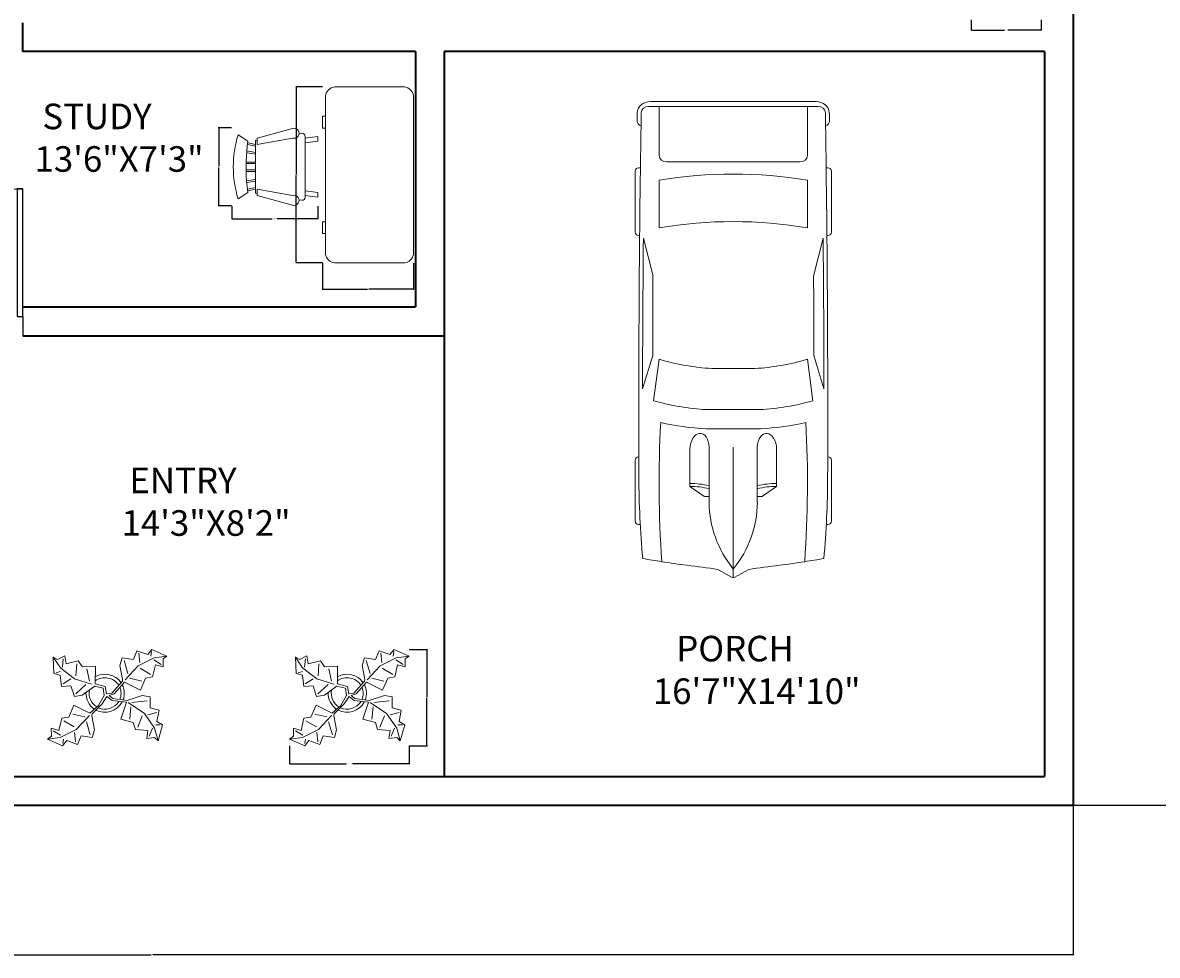
# Model space of a CAD drawing. Units: inches. Extents: x -1138 to 192, y 31 to 760.
# Tile 2 of 6: x -843 to -488, y 31 to 323. Entities that reach past the tile are written whole.
import ezdxf

# ---------------------------------------------------------------- set-up
doc = ezdxf.new("R2010")
doc.units = ezdxf.units.IN
doc.header["$MEASUREMENT"] = 0
for name, color, linetype, lineweight in [('A-ANNO-DIMS', 2, 'Continuous', 18), ('A-AREA-IDEN', 7, 'Continuous', 18), ('A-DOOR', 3, 'Continuous', 25), ('A-FURN', 8, 'Continuous', 18), ('A-SITE-VEHI', 8, 'Continuous', 13), ('A-WALL', 7, 'Continuous', 35), ('L-PLNT', 94, 'Continuous', 18)]:
    doc.layers.add(name, color=color, linetype=linetype, lineweight=lineweight)
doc.styles.get("Standard").update_dxf_attribs({"font": 'arial.ttf'})
doc.dimstyles.get("Standard").update_dxf_attribs({"dimtxt": 0.18, "dimasz": 0.18, "dimexe": 0.18, "dimexo": 0.0625, "dimgap": 0.09, "dimtad": 0, "dimtih": 1, "dimtoh": 1, "dimdec": 1, "dimzin": 0, "dimdsep": 46, "dimlunit": 4, "dimtxsty": 'Standard', "dimcen": 0.09, "dimadec": 0, "dimazin": 0, "dimtfac": 1, "dimtdec": 1, "dimtofl": 0, "dimtmove": 0, "dimatfit": 3, "dimfxl": 1, "dimtolj": 1, "dimtzin": 0, "dimarcsym": 0})

# ---------------------------------------------------------------- blocks, each defined once
blk = doc.blocks.new('*U9')
for p, q in [((0, 0), (0, -6)), ((40, 0), (40, -6))]:
    blk.add_line(p, q)
blk.add_lwpolyline([(0, 0), (0, 40), (1.75, 40), (1.75, 0)], close=True)
blk.add_arc((0, 0), 40, 0, 90)
blk = doc.blocks.new('*U11')
for p, q in [((536, 950), (536, 936)), ((1182, 988), (568, 988)), ((1214, 950), (1214, 950)), ((3440, 942), (3440, 950)), ((3472, 988), (4087, 988)), ((4119, 950), (4119, 934)), ((1779, 801), (2195, 746)), ((2235, 810), (1899, 912)), ((3412, 904), (3030, 807)), ((4736, -851), (4736, 851)), ((4785, -832), (4785, 832)), ((3516, 746), (3994, 746)), ((4736, 746), (4242, 746)), ((4179, 670), (4179, -670)), ((820, 295), (918, 436)), ((918, 436), (1294, 436)), ((756, 241), (1313, 241)), ((816, 241), (816, 283)), ((1496, -274), (1496, 274)), ((1690, -267), (1690, 267)), ((4736, -267), (4736, 267)), ((83, 156), (3, 10)), ((2102, 216), (2102, -216)), ((0, 0), (1313, 0)), ((3, -10), (83, -156)), ((756, -241), (1313, -241)), ((816, -241), (816, -283)), ((820, -295), (918, -436)), ((918, -436), (1294, -436)), ((2195, -746), (1779, -801)), ((3994, -746), (3516, -746)), ((4242, -746), (4736, -746)), ((2235, -810), (1899, -912)), ((3412, -904), (3030, -807)), ((536, -950), (536, -936)), ((1182, -988), (568, -988)), ((1214, -950), (1214, -950)), ((3440, -942), (3440, -950)), ((3472, -988), (4087, -988)), ((4119, -950), (4119, -934))]:
    blk.add_line(p, q)
for centre, major_axis, ratio, start_param, end_param in [((1046, -12468), (0, 13417), 0.842304, 0.00281, 0.075598), ((568, 950), (0, -37.6), 0.842304, 3.141593, 4.712389), ((1638, -268113), (0, 269063), 0.842304, -0.013397, 0.002797), ((1182, 950), (0, 37.6), 0.842304, -1.570796, 0), ((3472, 950), (0, -37.6), 0.842304, 3.141593, 4.712389), ((4087, 950), (0, 37.6), 0.842304, -1.570796, 0), ((4588, 910), (0, 56.4), 0.842304, -0.013017, 1.249894), ((1638, -268131), (0, 269121), 0.842304, -0.013397, -0.013017), ((4673, 851), (0, -75.2), 0.842304, 1.570796, 3.128196), ((4673, 832), (0, -133), 0.842304, 1.570796, 3.128196), ((6757, -699), (0, 7958), 0.842304, 1.367076, 1.39176), ((3436, 137), (0, 2077), 0.842304, 1.245306, 1.50788), ((1638, -268113), (0, -269025), 0.842304, 3.133765, 3.140441), ((2433, -93125), (0, -93935), 0.842304, 3.134049, 3.144098), ((6583, -699), (0, -7755), 0.842304, 4.528606, 4.561838), ((952, -15087), (0, -15833), 0.842304, 3.096046, 3.200911), ((3414, 137), (0, -2280), 0.842304, 4.449482, 4.652344), ((3800, 71), (0, -2021), 0.842304, 4.372215, 4.640744), ((434, 0), (0, 3734), 0.842304, 4.511394, 4.913384), ((912, 0), (0, 3734), 0.842304, 4.511394, 4.913384), ((4242, 670), (0, 75.2), 0.842304, 0, 1.570796), ((-5194, 1331), (0, -6374), 0.842304, 1.385369, 1.434372), ((331, 432), (0, 696), 0.842304, 4.435146, 4.718221), ((361, 432), (0, 696), 0.842304, 4.435146, 4.718221), ((1290, 339), (161, -9), 0.603834, -1.395552, 1.581315), ((756, -1185), (0, 1427), 0.842304, 0, 0.590319), ((832, 283), (0, 18.8), 0.842304, 0.879714, 1.570796), ((16, 0), (0, -18.8), 0.842304, 4.131459, 5.293319), ((756, 1185), (0, 1427), 0.842304, 2.551274, 3.141593), ((-5194, -1331), (0, 6374), 0.842304, -1.434372, -1.385369), ((3800, -71), (0, -2021), 0.842304, -1.499151, -1.230623), ((832, -283), (0, -18.8), 0.842304, 4.712389, 5.403472), ((331, -432), (0, -696), 0.842304, 1.564964, 1.848039), ((361, -432), (0, -696), 0.842304, 1.564964, 1.848039), ((3414, -137), (0, -2280), 0.842304, -1.510751, -1.307889), ((3436, -137), (0, -2077), 0.842304, -1.50788, -1.245306), ((6583, 699), (0, 7755), 0.842304, 1.721348, 1.754579), ((4242, -670), (0, -75.2), 0.842304, 4.712389, 6.283185), ((6757, 699), (0, 7958), 0.842304, 1.749832, 1.774517), ((952, 15087), (0, -15833), 0.842304, -0.059319, 0.045547), ((1046, 12468), (0, -13417), 0.842304, -0.075598, -0.00281), ((1638, 268113), (0, -269025), 0.842304, 0.001152, 0.007828), ((2433, 93125), (0, -93935), 0.842304, -0.002505, 0.007544), ((4673, -851), (0, 75.2), 0.842304, 3.15499, 4.712389), ((4673, -832), (0, -133), 0.842304, 0.013397, 1.570796), ((568, -950), (0, 37.6), 0.842304, 1.570796, 3.141593), ((1638, 268113), (0, 269063), 0.842304, 3.138796, 3.15499), ((1182, -950), (0, -37.6), 0.842304, 0, 1.570796), ((3472, -950), (0, -37.6), 0.842304, -1.570796, 0), ((4087, -950), (0, 37.6), 0.842304, 3.141593, 4.712389), ((4588, -910), (0, -56.4), 0.842304, -1.249894, 0.013017), ((1638, 268131), (0, 269121), 0.842304, 3.15461, 3.15499)]:
    blk.add_ellipse(centre, major_axis=major_axis, ratio=ratio, start_param=start_param, end_param=end_param)
at = {"extrusion": (0, 0, -1)}
blk.add_ellipse((1290, -339), major_axis=(161, 9), ratio=0.603834, start_param=-1.395552, end_param=1.581315, dxfattribs=at)
blk = doc.blocks.new('Plant - Rubber or Philodendron')
for p, q in [((-16.2005, 11.4774), (-13.9899, 8.1064)), ((-16.2005, 11.4774), (-14.8639, 10.7964)), ((-16.0159, 6.3329), (-16.2005, 11.4774)), ((-14.8639, 10.7964), (-12.6195, 11.8975)), ((-13.3174, 8.325), (-13.0735, 11.0065)), ((-12.6195, 11.8975), (-12.1909, 9.4345)), ((4.6914, 8.8812), (5.3859, 11.2828)), ((5.3859, 11.2828), (8.8871, 10.7908)), ((8.8871, 10.7908), (9.9809, 13.4933)), ((9.9809, 13.4933), (13.3837, 12.301)), ((15.3859, 11.3055), (10.3916, 8.7942)), ((10.5828, 12.6946), (10.8893, 9.7953)), ((13.3837, 12.301), (14.68, 13.9039)), ((14.5816, 13.2037), (14.3848, 11.8033)), ((14.68, 13.9039), (19.3848, 11.8146)), ((19.3848, 11.8146), (15.3859, 11.3055)), ((19.3848, 11.8146), (18.1868, 10.9119)), ((18.1868, 10.9119), (18.1925, 8.4119)), ((-13.9899, 8.1064), (-9.5434, 4.7185)), ((-12.1909, 9.4345), (-8.3829, 10.3)), ((-8.8369, 9.409), (-9.0894, 5.6095)), ((-8.3829, 10.3), (-7.0549, 8.501)), ((-7.0549, 8.501), (-3.0284, 8.6941)), ((-4.8529, 4.012), (-5.7184, 7.82)), ((-3.0284, 8.6941), (-3.0709, 3.1041)), ((4.6914, 8.8812), (5.5014, 4.4831)), ((5.9878, 10.4842), (7.1971, 6.3869)), ((10.3916, 8.7942), (6.2847, 4.4028)), ((14.2977, 6.1031), (10.9934, 7.9956)), ((15.7909, 9.1065), (14.8995, 5.3044)), ((15.2875, 10.6053), (17.5907, 9.2105)), ((18.1925, 8.4119), (15.7909, 9.1065)), ((-14.0069, 5.8704), (-16.0159, 6.3329)), ((-15.3434, 6.5514), (-13.9984, 6.9884)), ((-13.5868, 2.2894), (-14.0069, 5.8704)), ((-13.1329, 3.1804), (-10.6614, 4.727)), ((-9.5434, 4.7185), (-4.1917, 2.9888)), ((2.1141, 0.2298), (5.4346, 3.9146)), ((6.1032, 3.6844), (2.8262, -0.031)), ((5.4346, 3.9146), (5.5014, 4.4831)), ((11.1089, 1.1958), (6.1032, 3.6844)), ((7.7005, 4.8881), (11.5025, 3.9967)), ((12.7005, 4.8994), (11.1089, 1.1958)), ((14.8995, 5.3044), (12.7005, 4.8994)), ((-10.6784, 2.491), (-13.5868, 2.2894)), ((-9.5858, -0.8715), (-10.6784, 2.491)), ((-9.1318, 0.0195), (-5.9793, 2.9025)), ((-7.1228, -0.443), (-3.5248, 2.2131)), ((-3.5248, 2.2131), (-3.3011, 2.4355)), ((-3.3011, 2.4355), (-0.5306, 1.7947)), ((-3.0709, 3.1041), (0.0797, 2.3163)), ((-0.5306, 1.7947), (-0.2255, -0.5527)), ((-0.5306, 1.7947), (-0.5306, 1.7947)), ((0.0797, 2.3163), (0.4866, -0.031)), ((0.4866, -0.031), (2.1141, 0.2298)), ((-7.1228, -0.443), (-9.5858, -0.8715)), ((-4.0579, -6.2781), (-0.9375, -3.1608)), ((-2.019, -3.6148), (-0.2255, -0.5527)), ((-0.9375, -3.1608), (0.5883, -0.8135)), ((0.5883, -0.8135), (2.2447, -2.0916)), ((2.8262, -0.031), (1.3003, -0.5527)), ((1.3003, -0.5527), (2.4193, -1.4655)), ((2.2447, -2.0916), (6.7108, -2.6626)), ((2.4193, -1.4655), (6.895, -2.1175)), ((4.943, -7.9659), (6.7108, -2.6626)), ((11.6605, -0.5413), (6.895, -2.1175)), ((12.3677, -6.1981), (7.219, -2.6772)), ((8.3544, -2.7453), (13.1973, -2.1704)), ((11.6605, -0.5413), (14.1354, -0.8948)), ((14.1354, -0.8948), (14.1354, -4.4304)), ((-11.3237, -7.2629), (-9.7321, -3.5593)), ((-6.3237, -7.2516), (-10.1257, -6.3602)), ((-9.7321, -3.5593), (-4.7264, -6.0479)), ((-9.0148, -11.1577), (-4.9047, -6.8122)), ((-2.019, -3.6148), (-4.7264, -6.0479)), ((-4.1246, -6.8466), (-4.0579, -6.2781)), ((-3.3146, -11.2447), (-4.1246, -6.8466)), ((8.125, -4.0768), (7.7715, -7.9659)), ((10.2463, -10.4408), (11.6605, -6.9053)), ((15.5496, -10.7943), (12.3677, -6.1981)), ((16.2567, -5.8446), (13.4283, -6.5517)), ((14.1354, -4.4304), (16.9638, -5.1375)), ((16.9638, -5.1375), (16.2567, -8.673)), ((-14.4141, -11.4699), (-13.5228, -7.6679)), ((-13.5228, -7.6679), (-11.3237, -7.2629)), ((-12.921, -8.4665), (-9.6166, -10.359)), ((-4.611, -12.8477), (-5.8203, -8.7504)), ((8.8321, -9.0266), (4.943, -7.9659)), ((9.5392, -11.1479), (8.8321, -9.0266)), ((17.3174, -9.7337), (15.9032, -9.7337)), ((16.2567, -8.673), (18.0245, -9.7337)), ((18.0245, -9.7337), (16.6103, -14.6834)), ((-18.008, -14.1781), (-16.8101, -13.2754)), ((-18.008, -14.1781), (-14.0091, -13.669)), ((-13.3032, -16.2674), (-18.008, -14.1781)), ((-16.8157, -10.7754), (-14.4141, -11.4699)), ((-16.8101, -13.2754), (-16.8157, -10.7754)), ((-13.9107, -12.9688), (-16.2139, -11.574)), ((-14.0091, -13.669), (-9.0148, -11.1577)), ((-13.2048, -15.5672), (-13.008, -14.1668)), ((-9.206, -15.0581), (-9.5126, -12.1588)), ((-7.5103, -13.1543), (-8.6042, -15.8568)), ((-4.0092, -13.6463), (-7.5103, -13.1543)), ((-3.3146, -11.2447), (-4.0092, -13.6463)), ((13.4283, -11.5015), (9.5392, -11.1479)), ((13.0748, -13.9763), (13.4283, -11.5015)), ((15.5496, -13.6228), (13.0748, -13.9763)), ((14.8425, -10.7943), (13.7819, -13.2692)), ((16.6103, -14.6834), (15.5496, -10.7943)), ((16.6103, -14.6834), (15.5496, -13.6228)), ((-12.0069, -14.6645), (-13.3032, -16.2674)), ((-8.6042, -15.8568), (-12.0069, -14.6645))]:
    blk.add_line(p, q)
for centre, radius, start, end in [((0, 0), 6.1275, 34.37569, 120.1028), ((-0.0601, -0.2075), 5.2461, 33.82192, 124.9414), ((0.0308, 0.1664), 6, 178.6147, 235.1169), ((0.0308, 0.1664), 5, 168.1647, 238.6725), ((-0.2664, 0.1682), 5.2775, 338.4094, 20.03007), ((-0.098, 0.1364), 6.1288, 341.2017, 26.09184), ((-0.0234, 0.3825), 6.1492, 242.5812, 331.2714), ((-0.1102, 0.4886), 5.2883, 247.3711, 327.472)]:
    blk.add_arc(centre, radius, start, end)
blk = doc.blocks.new('Desk - 30 x 60 in.')
for p, q in [((-26.999995, 0), (26.999995, 0)), ((-29.999995, -27), (-29.999995, -3)), ((29.999995, -3), (29.999995, -27)), ((26.999995, -30), (-26.999995, -30)), ((-20.000005, -30), (-20.000005, -31)), ((-16.000005, -31), (-16.000005, -30)), ((15.999995, -31), (15.999995, -30)), ((19.999995, -30), (19.999995, -31)), ((-20.000005, -31), (-16.000005, -31)), ((19.999995, -31), (15.999995, -31))]:
    blk.add_line(p, q)
for centre, start, end in [((-26.499995, -3.5), 98.1301, 171.8699), ((26.499995, -3.5), 8.130102, 81.8699), ((-26.499995, -26.5), 188.1301, 261.8699), ((26.499995, -26.5), 278.1301, 351.8699)]:
    blk.add_arc(centre, 3.535534, start, end)
blk = doc.blocks.new('Chair - Rocking')
for p, q in [((-8, -4.5), (-10, -1.5)), ((8, -4.5), (10, -1.5)), ((-8.23428, -6.99939), (-8.3093, -7.47958)), ((-8.23041, -7), (8.23915, -7)), ((-7.5, -4.5), (-7, -7)), ((-6.5, -7), (-7.02225, -4.43)), ((-4.5, -7), (-4.96674, -4.19951)), ((-4, -7), (-4.40532, -4.16272)), ((-1.5, -4.05012), (-1.5, -7)), ((-1, -7), (-1, -4.05012)), ((1, -7), (1, -4.04655)), ((1.5, -4.05012), (1.5, -7)), ((4, -7), (4.40187, -4.18694)), ((4.5, -7), (4.96761, -4.19437)), ((6.5, -7), (7, -4.4057)), ((7.5, -4.5), (7, -7)), ((8.31071, -7.48854), (8.23449, -7.00073)), ((-9, -7.5), (-12, -18.49999)), ((-7, -7.5), (-9, -7.5)), ((-9, -18.49999), (-7, -7.5)), ((7, -7.5), (9, -7.5)), ((9, -18.49999), (7, -7.5)), ((9, -7.5), (12, -18.49999)), ((-10.36644, -20.64523), (-10.5, -21.49999)), ((10.5, -21.49999), (10.3575, -20.58798)), ((-9, -22.49999), (-9.5, -26.49999)), ((0, -22.49999), (-9.5, -22.49999)), ((-8, -26.49999), (-7.5, -22.49999)), ((0, -22.49999), (9.5, -22.49999)), ((8, -26.49999), (7.5, -22.49999)), ((9, -22.49999), (9.5, -26.49999)), ((-9.5, -26.49999), (-8, -26.49999)), ((9.5, -26.49999), (8, -26.49999))]:
    blk.add_line(p, q)
for centre, radius, start, end in [((0, -34.08333), 34.08333, 72.93847, 107.0615), ((0, -68.25004), 64.25, 93.92211, 97.15267), ((0, -68.25004), 64.25, 82.84733, 93.92211), ((-10.5, -18.99999), 1.58114, 161.5651, 18.43495), ((10.5, -18.99999), 1.58114, 161.5651, 18.43495), ((-9.5, -21.49999), 1, 180, 270), ((9.5, -21.49999), 1, 270, 0)]:
    blk.add_arc(centre, radius, start, end)
blk = doc.blocks.new('*D55')
at = {"layer": 'A-ANNO-DIMS', "color": 0, "lineweight": -2, "transparency": 16777216}
for p, q in [((-759.52, 96.35), (-759.52, 90.63)), ((-722.12, 96.35), (-722.12, 90.63)), ((-759.34, 90.81), (-741.78, 90.81)), ((-722.3, 90.81), (-739.86, 90.81))]:
    blk.add_line(p, q, dxfattribs=at)
at = {"layer": 'A-ANNO-DIMS', "color": 0, "transparency": 16777216}
for points in [[(-759.34, 90.84), (-759.34, 90.78), (-759.52, 90.81)], [(-722.3, 90.84), (-722.3, 90.78), (-722.12, 90.81)]]:
    blk.add_solid(points, dxfattribs=at)
at = {"layer": 'Defpoints', "color": 0, "transparency": 16777216}
for p in [(-759.52, 96.42), (-722.12, 96.42), (-722.12, 90.81)]:
    blk.add_point(p, dxfattribs=at)
at = {"layer": 'A-ANNO-DIMS', "color": 0, "transparency": 16777216, "insert": (-740.82, 90.81), "char_height": 0.18, "attachment_point": 5}
blk.add_mtext('\\A1;PLANT 37 TYP.', dxfattribs=at)
blk = doc.blocks.new('*D56')
at = {"layer": 'A-ANNO-DIMS', "color": 0, "lineweight": -2, "transparency": 16777216}
for p, q in [((-722.06, 126.59), (-716.33, 126.59)), ((-716.51, 126.41), (-716.51, 111.68)), ((-716.51, 96.6), (-716.51, 111.32)), ((-722.06, 96.42), (-716.33, 96.42))]:
    blk.add_line(p, q, dxfattribs=at)
at = {"layer": 'A-ANNO-DIMS', "color": 0, "transparency": 16777216}
for points in [[(-716.54, 126.41), (-716.48, 126.41), (-716.51, 126.59)], [(-716.54, 96.6), (-716.48, 96.6), (-716.51, 96.42)]]:
    blk.add_solid(points, dxfattribs=at)
at = {"layer": 'Defpoints', "color": 0, "transparency": 16777216}
for p in [(-722.12, 126.59), (-716.51, 126.59), (-722.12, 96.42)]:
    blk.add_point(p, dxfattribs=at)
at = {"layer": 'A-ANNO-DIMS', "color": 0, "transparency": 16777216, "insert": (-716.51, 111.5), "char_height": 0.18, "attachment_point": 5}
blk.add_mtext('\\A1;30 TYP.', dxfattribs=at)
blk = doc.blocks.new('*D64')
at = {"layer": 'A-ANNO-DIMS', "color": 0, "lineweight": -2, "transparency": 16777216}
for p, q in [((-546.05, 323.73), (-546.05, 320.32)), ((-524.13, 323.73), (-524.13, 320.32)), ((-545.87, 320.5), (-535.62, 320.5)), ((-524.31, 320.5), (-534.56, 320.5))]:
    blk.add_line(p, q, dxfattribs=at)
at = {"layer": 'A-ANNO-DIMS', "color": 0, "transparency": 16777216}
for points in [[(-545.87, 320.53), (-545.87, 320.47), (-546.05, 320.5)], [(-524.31, 320.53), (-524.31, 320.47), (-524.13, 320.5)]]:
    blk.add_solid(points, dxfattribs=at)
at = {"layer": 'Defpoints', "color": 0, "transparency": 16777216}
for p in [(-546.05, 323.79), (-524.13, 323.79), (-524.13, 320.5)]:
    blk.add_point(p, dxfattribs=at)
at = {"layer": 'A-ANNO-DIMS', "color": 0, "transparency": 16777216, "insert": (-535.09, 320.5), "char_height": 0.18, "attachment_point": 5}
blk.add_mtext('\\A1;22 TYP.', dxfattribs=at)
blk = doc.blocks.new('*D77')
at = {"layer": 'A-ANNO-DIMS', "color": 0, "lineweight": -2, "transparency": 16777216}
for p, q in [((-749.24, 302.69), (-757.62, 302.69)), ((-757.44, 302.51), (-757.44, 275.33)), ((-757.44, 247.79), (-757.44, 274.97)), ((-749.24, 247.61), (-757.62, 247.61))]:
    blk.add_line(p, q, dxfattribs=at)
at = {"layer": 'A-ANNO-DIMS', "color": 0, "transparency": 16777216}
for points in [[(-757.47, 302.51), (-757.41, 302.51), (-757.44, 302.69)], [(-757.47, 247.79), (-757.41, 247.79), (-757.44, 247.61)]]:
    blk.add_solid(points, dxfattribs=at)
at = {"layer": 'Defpoints', "color": 0, "transparency": 16777216}
for p in [(-749.18, 302.69), (-757.44, 247.61), (-749.18, 247.61)]:
    blk.add_point(p, dxfattribs=at)
at = {"layer": 'A-ANNO-DIMS', "color": 0, "transparency": 16777216, "insert": (-757.44, 275.15), "char_height": 0.18, "attachment_point": 5}
blk.add_mtext('\\A1;DESK 55', dxfattribs=at)
blk = doc.blocks.new('*D78')
at = {"layer": 'A-ANNO-DIMS', "color": 0, "lineweight": -2, "transparency": 16777216}
for p, q in [((-749.18, 247.55), (-749.18, 239.17)), ((-720.72, 247.55), (-720.72, 239.17)), ((-749, 239.35), (-735.17, 239.35)), ((-720.9, 239.35), (-734.73, 239.35))]:
    blk.add_line(p, q, dxfattribs=at)
at = {"layer": 'A-ANNO-DIMS', "color": 0, "transparency": 16777216}
for points in [[(-749, 239.38), (-749, 239.32), (-749.18, 239.35)], [(-720.9, 239.38), (-720.9, 239.32), (-720.72, 239.35)]]:
    blk.add_solid(points, dxfattribs=at)
at = {"layer": 'Defpoints', "color": 0, "transparency": 16777216}
for p in [(-749.18, 247.61), (-720.72, 247.61), (-720.72, 239.35)]:
    blk.add_point(p, dxfattribs=at)
at = {"layer": 'A-ANNO-DIMS', "color": 0, "transparency": 16777216, "insert": (-734.95, 239.35), "char_height": 0.18, "attachment_point": 5}
blk.add_mtext('\\A1;28', dxfattribs=at)
blk = doc.blocks.new('*D79')
at = {"layer": 'A-ANNO-DIMS', "color": 0, "lineweight": -2, "transparency": 16777216}
for p, q in [((-777.66, 265.42), (-777.66, 261.25)), ((-750.66, 265.42), (-750.66, 261.25)), ((-777.48, 261.43), (-764.95, 261.43)), ((-750.84, 261.43), (-763.38, 261.43))]:
    blk.add_line(p, q, dxfattribs=at)
at = {"layer": 'A-ANNO-DIMS', "color": 0, "transparency": 16777216}
for points in [[(-777.48, 261.46), (-777.48, 261.4), (-777.66, 261.43)], [(-750.84, 261.46), (-750.84, 261.4), (-750.66, 261.43)]]:
    blk.add_solid(points, dxfattribs=at)
at = {"layer": 'Defpoints', "color": 0, "transparency": 16777216}
for p in [(-777.66, 265.48), (-750.66, 265.48), (-777.66, 261.43)]:
    blk.add_point(p, dxfattribs=at)
at = {"layer": 'A-ANNO-DIMS', "color": 0, "transparency": 16777216, "insert": (-764.16, 261.43), "char_height": 0.18, "attachment_point": 5}
blk.add_mtext('\\A1;ROCKER 27', dxfattribs=at)
blk = doc.blocks.new('*D80')
at = {"layer": 'A-ANNO-DIMS', "color": 0, "lineweight": -2, "transparency": 16777216}
for p, q in [((-777.73, 289.91), (-781.89, 289.91)), ((-781.71, 289.73), (-781.71, 277.88)), ((-781.71, 265.66), (-781.71, 277.52)), ((-777.73, 265.48), (-781.89, 265.48))]:
    blk.add_line(p, q, dxfattribs=at)
at = {"layer": 'A-ANNO-DIMS', "color": 0, "transparency": 16777216}
for points in [[(-781.74, 289.73), (-781.68, 289.73), (-781.71, 289.91)], [(-781.74, 265.66), (-781.68, 265.66), (-781.71, 265.48)]]:
    blk.add_solid(points, dxfattribs=at)
at = {"layer": 'Defpoints', "color": 0, "transparency": 16777216}
for p in [(-781.71, 289.91), (-777.66, 289.91), (-777.66, 265.48)]:
    blk.add_point(p, dxfattribs=at)
at = {"layer": 'A-ANNO-DIMS', "color": 0, "transparency": 16777216, "insert": (-781.71, 277.7), "char_height": 0.18, "attachment_point": 5}
blk.add_mtext('\\A1;24', dxfattribs=at)
blk = doc.blocks.new('*D85')
at = {"layer": 'A-ANNO-DIMS', "color": 0, "lineweight": -2, "transparency": 16777216}
for p, q in [((-1091.13, 77.75), (-1091.13, 30.82)), ((-514.13, 77.75), (-514.13, 30.82)), ((-1090.95, 31), (-802.92, 31)), ((-514.31, 31), (-802.34, 31))]:
    blk.add_line(p, q, dxfattribs=at)
at = {"layer": 'A-ANNO-DIMS', "color": 0, "transparency": 16777216}
for points in [[(-1090.95, 31.03), (-1090.95, 30.97), (-1091.13, 31)], [(-514.31, 31.03), (-514.31, 30.97), (-514.13, 31)]]:
    blk.add_solid(points, dxfattribs=at)
at = {"layer": 'Defpoints', "color": 0, "transparency": 16777216}
for p in [(-1091.13, 77.81), (-514.13, 77.81), (-514.13, 31)]:
    blk.add_point(p, dxfattribs=at)
at = {"layer": 'A-ANNO-DIMS', "color": 0, "transparency": 16777216, "insert": (-802.63, 31), "char_height": 0.18, "attachment_point": 5}
blk.add_mtext('\\A1;577', dxfattribs=at)
blk = doc.blocks.new('*D86')
at = {"layer": 'A-ANNO-DIMS', "color": 0, "lineweight": -2, "transparency": 16777216}
for p, q in [((-514.07, 700.81), (-467.14, 700.81)), ((-467.32, 700.63), (-467.32, 389.49)), ((-467.32, 77.99), (-467.32, 389.13)), ((-514.07, 77.81), (-467.14, 77.81))]:
    blk.add_line(p, q, dxfattribs=at)
at = {"layer": 'A-ANNO-DIMS', "color": 0, "transparency": 16777216}
for points in [[(-467.35, 700.63), (-467.29, 700.63), (-467.32, 700.81)], [(-467.35, 77.99), (-467.29, 77.99), (-467.32, 77.81)]]:
    blk.add_solid(points, dxfattribs=at)
at = {"layer": 'Defpoints', "color": 0, "transparency": 16777216}
for p in [(-514.13, 700.81), (-467.32, 700.81), (-514.13, 77.81)]:
    blk.add_point(p, dxfattribs=at)
at = {"layer": 'A-ANNO-DIMS', "color": 0, "transparency": 16777216, "insert": (-467.32, 389.31), "char_height": 0.18, "attachment_point": 5}
blk.add_mtext('\\A1;623', dxfattribs=at)

msp = doc.modelspace()

# ---------------------------------------------------------------- linework, layer by layer
at = {"layer": 'A-WALL'}
for p, q in [((-514.133, 371.813), (-514.133, 77.813)), ((-843.133, 313.813), (-843.133, 322.813)), ((-720.133, 313.813), (-843.133, 313.813)), ((-720.133, 313.813), (-720.133, 233.813)), ((-523.133, 313.813), (-711.133, 313.813)), ((-711.133, 313.813), (-711.133, 224.813)), ((-523.133, 313.813), (-523.133, 86.813)), ((-843.133, 233.813), (-720.133, 233.813)), ((-843.133, 224.813), (-711.133, 224.813)), ((-711.133, 224.813), (-711.133, 86.813)), ((-923.133, 86.813), (-523.133, 86.813)), ((-1091.133, 77.813), (-514.133, 77.813))]:
    msp.add_line(p, q, dxfattribs=at)

# ---------------------------------------------------------------- block references
at = {"layer": 'A-DOOR', "xscale": -1}
msp.add_blockref('*U9', (-843.133, 230.813), dxfattribs=at)
at = {"layer": 'A-FURN', "xscale": 0.9179024525527003, "yscale": 0.9179024525527003, "zscale": 0.9179024525527003, "rotation": 270}
msp.add_blockref('Desk - 30 x 60 in.', (-720.725, 275.15), dxfattribs=at)
at = {"layer": 'A-FURN', "rotation": 90}
msp.add_blockref('Chair - Rocking', (-777.163, 277.697), dxfattribs=at)
at = {"layer": 'A-SITE-VEHI', "xscale": 0.0311530432293533, "yscale": 0.0311530432293533, "zscale": 0.0311530432293533, "rotation": 90}
msp.add_blockref('*U11', (-620.566, 149.039), dxfattribs=at)
at = {"layer": 'L-PLNT'}
for p in [(-817.35, 112.684), (-741.507, 112.684)]:
    msp.add_blockref('Plant - Rubber or Philodendron', p, dxfattribs=at)

# ---------------------------------------------------------------- texts
at = {"layer": 'A-AREA-IDEN', "char_height": 8, "attachment_point": 1}
for s, insert in [(' STUDY\\P13\'6"X7\'3"', (-839.42, 297.477)), (' ENTRY\\P14\'3"X8\'2"', (-812.167, 183.505)), ('   PORCH\\P16\'7"X14\'10"', (-645.765, 130.841))]:
    msp.add_mtext_dynamic_manual_height_columns(s, width=126.58932, gutter_width=1, heights=[0], dxfattribs=dict(at, insert=insert))

# ---------------------------------------------------------------- dimensions: what is measured, and where the dimension line sits
at = {"layer": 'A-ANNO-DIMS'}
for base, p1, p2, picture, middle in [((-467.318, 700.813), (-514.133, 77.813), (-514.133, 700.813), '*D86', (-467.318, 389.313)), ((-781.713, 289.915), (-777.663, 265.48), (-777.663, 289.915), '*D80', (-781.713, 277.697))]:
    dim = msp.add_linear_dim(base=base, p1=p1, p2=p2, angle=90, dimstyle='Standard', override={"dimdec": 0, "dimlfac": 1, "dimrnd": 0, "dimzin": 0, "dimdsep": 46, "dimlunit": 2}, dxfattribs=at)
    dim.commit()
    dim.dimension.update_dxf_attribs({"geometry": picture, "text_midpoint": middle})
for base, p1, p2, text, picture, middle in [((-524.132, 320.501), (-546.047, 323.789), (-524.132, 323.789), '<> TYP.', '*D64', (-535.089, 320.501)), ((-722.123, 90.808), (-759.515, 96.417), (-722.123, 96.417), 'PLANT <> TYP.', '*D55', (-740.819, 90.808))]:
    dim = msp.add_linear_dim(base=base, p1=p1, p2=p2, text=text, dimstyle='Standard', override={"dimdec": 0, "dimlfac": 1, "dimrnd": 0, "dimzin": 0, "dimdsep": 46, "dimlunit": 2}, dxfattribs=at)
    dim.commit()
    dim.dimension.update_dxf_attribs({"geometry": picture, "text_midpoint": middle})
for base, p1, p2, angle, text, picture, middle in [((-757.441, 247.613), (-749.18, 302.687), (-749.18, 247.613), 270, 'DESK <>', '*D77', (-757.441, 275.15)), ((-777.663, 261.43), (-750.663, 265.48), (-777.663, 265.48), 180, 'ROCKER <>', '*D79', (-764.163, 261.43)), ((-716.514, 126.588), (-722.123, 96.417), (-722.123, 126.588), 90, '<> TYP.', '*D56', (-716.514, 111.502))]:
    dim = msp.add_linear_dim(base=base, p1=p1, p2=p2, angle=angle, text=text, dimstyle='Standard', override={"dimdec": 0, "dimlfac": 1, "dimrnd": 0, "dimzin": 0, "dimdsep": 46, "dimlunit": 2}, dxfattribs=at)
    dim.commit()
    dim.dimension.update_dxf_attribs({"geometry": picture, "text_midpoint": middle})
for base, p1, p2, picture, middle in [((-720.725, 239.352), (-749.18, 247.613), (-720.725, 247.613), '*D78', (-734.952, 239.352)), ((-514.133, 30.998), (-1091.133, 77.813), (-514.133, 77.813), '*D85', (-802.633, 30.998))]:
    dim = msp.add_linear_dim(base=base, p1=p1, p2=p2, dimstyle='Standard', override={"dimdec": 0, "dimlfac": 1, "dimrnd": 0, "dimzin": 0, "dimdsep": 46, "dimlunit": 2}, dxfattribs=at)
    dim.commit()
    dim.dimension.update_dxf_attribs({"geometry": picture, "text_midpoint": middle})

doc.saveas('drawing.dxf')
